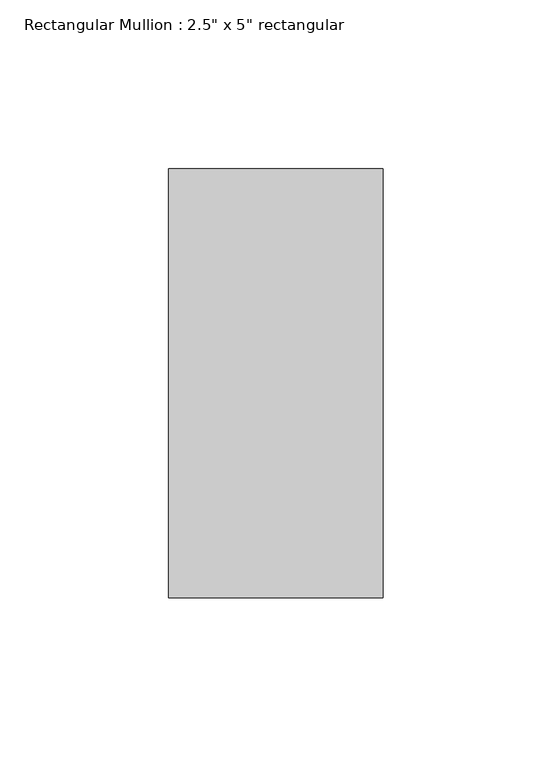
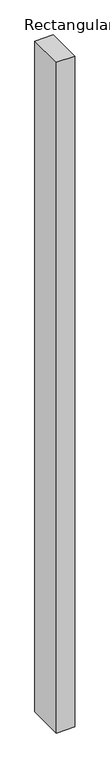
"""IFC4 building model written with IfcOpenShell, lengths in millimetres: member geometry."""

from ifc_helpers import new_model, si_unit, frame, origin, place, context, project, spatial, polyline, outline, extrude, source, transform, mapped, element, save


def member_189d47d0(model_context):
    return source(origin(), model_context, "Body", "SweptSolid", [
        extrude(outline(polyline([(31.75, 63.5), (31.75, -63.5), (-31.75, -63.5), (-31.75, 63.5), (31.75, 63.5)])), frame((0.0, 0.0, -2428.9640157), z_axis=(0.0, 0.0, 1.0), x_axis=(1.0, 0.0, 0.0)), (0.0, 0.0, 1.0), 2428.9640157),
    ])


if __name__ == "__main__":
    model = new_model("IFC4")
    model_context = context("Model", 3, world=origin())
    ifc_project = project(units=[si_unit("LENGTHUNIT", "METRE", prefix="MILLI")], contexts=[model_context])
    site = spatial("IfcSite", under=ifc_project)
    building = spatial("IfcBuilding", under=site)
    placement = place(None, origin())
    member_shape = member_189d47d0(model_context)
    element("IfcMember", 1, ObjectType="Rectangular Mullion : 2.5\" x 5\" rectangular", at=placement, inside=building, context=model_context, shape_type="MappedRepresentation", body=[
        mapped(member_shape, transform((0.0, 0.0, 0.0), x_axis=(1.0, 0.0, 0.0), y_axis=(0.0, 1.0, 0.0), z_axis=(0.0, 0.0, 1.0))),
    ])
    save(model, "model.ifc")

# Revit data of these elements
# Type "Rectangular Mullion : 2.5\" x 5\" rectangular"
#   built-in parameter 1007304 = 0.416667 (stored number, unit not read)
#   built-in parameter 1007301 = 0.104167 (stored number, unit not read)
#   built-in parameter 1007300 = 0.104167 (stored number, unit not read)
# Element 1 (IfcMember, "Rectangular Mullion : 2.5\" x 5\" rectangular")
#   Materials on its faces: "BLACK COLOUR"
# Materials
#   "BLACK COLOUR": class "Generic", colour RGB 120 120 120, transparency 0, Cost = 0
